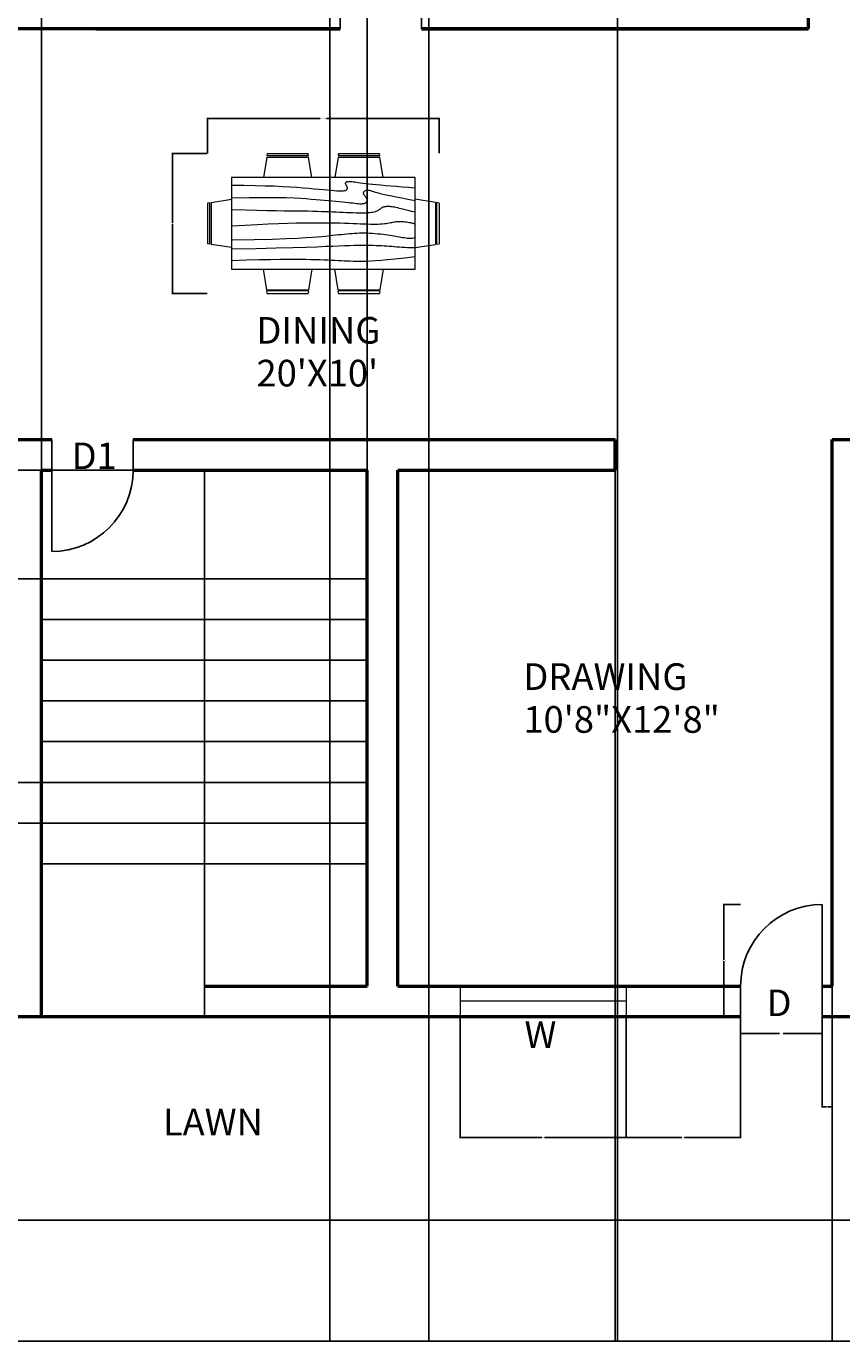
# Model space of a CAD drawing. Units: feet. Extents: x 1544 to 2324, y 1847 to 2475.
# Tile 2 of 4: x 1821 to 2061, y 1847 to 2234. Entities that reach past the tile are written whole.
import ezdxf

# ---------------------------------------------------------------- set-up
doc = ezdxf.new("R2010")
doc.units = ezdxf.units.FT
for name, color, linetype, lineweight in [('A-ANNO-DIMS', 2, 'Continuous', 18), ('A-ANNO-TEXT', 7, 'Continuous', 18), ('A-AREA-IDEN', 7, 'Continuous', 20), ('A-DOOR', 4, 'Continuous', 25), ('A-FLOR-STRS', 7, 'Continuous', 25), ('A-FURN', 8, 'Continuous', 18), ('A-GLAZ', 4, 'Continuous', 18), ('A-WALL', 7, 'Continuous', 50), ('C-PROP', 3, 'Continuous', 25)]:
    doc.layers.add(name, color=color, linetype=linetype, lineweight=lineweight)
doc.styles.get("Standard").update_dxf_attribs({"font": 'arial.ttf'})
doc.dimstyles.get("Standard").update_dxf_attribs({"dimtxt": 0.18, "dimasz": 0.18, "dimexe": 0.18, "dimexo": 0.0625, "dimgap": 0.09, "dimtad": 0, "dimtih": 1, "dimtoh": 1, "dimdec": 4, "dimzin": 0, "dimdsep": 46, "dimtxsty": 'Standard', "dimcen": 0.09, "dimadec": 0, "dimazin": 0, "dimtfac": 1, "dimtdec": 4, "dimtofl": 0, "dimtmove": 0, "dimatfit": 3, "dimfxl": 1, "dimtolj": 1, "dimtzin": 0, "dimarcsym": 0})

# ---------------------------------------------------------------- blocks, each defined once
blk = doc.blocks.new('Dining Set - 36 x 72 in.')
for p, q in [((-22.2343, 26.00059), (-23.4847, 17.99762)), ((-22.2304, 26), (-5.7608, 26)), ((-22, 27.5), (-22.1562, 26.50042)), ((-5.8416, 26.5), (-22.1534, 26.5)), ((-22, 27.5), (-6, 27.5)), ((-5.8437, 26.49966), (-6, 27.5)), ((-4.5152, 17.99762), (-5.7655, 25.99926)), ((5.7657, 26.00059), (4.5153, 17.99762)), ((5.7696, 26), (22.2392, 26)), ((6, 27.5), (5.8438, 26.50042)), ((22.1584, 26.5), (5.8466, 26.5)), ((6, 27.5), (22, 27.5)), ((22.1563, 26.49966), (22, 27.5)), ((23.4848, 17.99762), (22.2345, 25.99926)), ((36, 18), (-36, 18)), ((-36, 18), (-36, -18)), ((36, -18), (36, 18)), ((-45.5, 8), (-44.5004, 8.15617)), ((-45.5, 8), (-45.5, -8)), ((-44.5, -8.15843), (-44.5, 8.15338)), ((-44.0006, 8.23428), (-35.9976, 9.48474)), ((-44, 8.23041), (-44, -8.23915)), ((44.0006, 8.23428), (35.9976, 9.48474)), ((44, 8.23041), (44, -8.23915)), ((44.5, -8.15843), (44.5, 8.15338)), ((45.5, 8), (44.5005, 8.15617)), ((45.5, 8), (45.5, -8)), ((-44.4997, -8.15631), (-45.5, -8)), ((-35.9976, -9.48476), (-43.9993, -8.2345)), ((35.9976, -9.48476), (43.9993, -8.2345)), ((44.4997, -8.15631), (45.5, -8)), ((-36, -18), (36, -18)), ((-22.2343, -26.0006), (-23.4847, -17.99762)), ((-4.5152, -17.99762), (-5.7655, -25.99928)), ((5.7657, -26.0006), (4.5153, -17.99762)), ((23.4848, -17.99762), (22.2345, -25.99928)), ((-22.2304, -26), (-5.7608, -26)), ((-22, -27.5), (-22.1562, -26.50044)), ((-5.8416, -26.5), (-22.1534, -26.5)), ((-22, -27.5), (-6, -27.5)), ((-5.8437, -26.49967), (-6, -27.5)), ((5.7696, -26), (22.2392, -26)), ((6, -27.5), (5.8438, -26.50044)), ((22.1584, -26.5), (5.8466, -26.5)), ((6, -27.5), (22, -27.5)), ((22.1563, -26.49967), (22, -27.5))]:
    blk.add_line(p, q)
for points in [[(-36, 15), (-31.1772, 14.97754), (-26.8079, 14.91406), (-22.8538, 14.81543), (-19.276, 14.6875), (-16.0362, 14.53613), (-13.0957, 14.36718), (-10.4159, 14.18652), (-7.9583, 14), (-5.6904, 13.81315), (-3.6035, 13.63021), (-1.6954, 13.45508), (0.0365, 13.29166), (1.5945, 13.14388), (2.9811, 13.01562), (4.1988, 12.9108), (5.25, 12.83333), (6.1393, 12.78613), (6.8802, 12.76823), (7.4883, 12.77767), (7.9792, 12.8125), (8.3685, 12.87077), (8.6719, 12.95052), (8.9049, 13.0498), (9.0833, 13.16666), (9.2205, 13.29899), (9.3216, 13.44401), (9.3895, 13.59879), (9.4271, 13.76041), (9.4373, 13.92594), (9.4232, 14.09245), (9.3875, 14.257), (9.3333, 14.41666), (9.2638, 14.56917), (9.1836, 14.71484), (9.0975, 14.85465), (9.0104, 14.98958), (8.9272, 15.1206), (8.8529, 15.2487), (8.7922, 15.37483), (8.75, 15.5), (8.7305, 15.62467), (8.7344, 15.74739), (8.7617, 15.86621), (8.8125, 15.97916), (8.8867, 16.08431), (8.9844, 16.17968), (9.1055, 16.26334), (9.25, 16.33333), (9.4189, 16.38802), (9.6172, 16.42708), (9.8506, 16.45052), (10.125, 16.45833), (10.4463, 16.45052), (10.8203, 16.42708), (11.2529, 16.38802), (11.75, 16.33333), (12.3184, 16.26318), (12.9694, 16.17838), (13.7151, 16.07991), (14.5677, 15.96875), (15.5395, 15.84586), (16.6426, 15.71224), (17.8893, 15.56884), (19.2917, 15.41666), (20.859, 15.25667), (22.5879, 15.08984), (24.4721, 14.91715), (26.5052, 14.73958), (28.6809, 14.5581), (30.9929, 14.3737), (33.4347, 14.18733), (36, 14)], [(-36, 10), (-28.9766, 10.14274), (-23.1725, 10.20442), (-18.4241, 10.19775), (-14.5677, 10.13541), (-11.4399, 10.03011), (-8.877, 9.89453), (-6.7154, 9.74137), (-4.7917, 9.58333), (-2.9698, 9.43082), (-1.2246, 9.28515), (0.4415, 9.14534), (2.026, 9.01041), (3.5266, 8.87939), (4.9408, 8.7513), (6.266, 8.62516), (7.5, 8.5), (8.6411, 8.37549), (9.6914, 8.2539), (10.6538, 8.13818), (11.5312, 8.03125), (12.3267, 7.93603), (13.043, 7.85547), (13.6831, 7.79248), (14.25, 7.75), (14.7471, 7.7303), (15.1797, 7.73307), (15.5537, 7.75732), (15.875, 7.80208), (16.1494, 7.86637), (16.3828, 7.94922), (16.5811, 8.04964), (16.75, 8.16666), (16.8944, 8.29915), (17.0143, 8.44531), (17.1089, 8.60319), (17.1771, 8.77083), (17.218, 8.94629), (17.2305, 9.1276), (17.2137, 9.31282), (17.1667, 9.5), (17.0895, 9.6875), (16.987, 9.875), (16.8649, 10.0625), (16.7292, 10.25), (16.5856, 10.4375), (16.4401, 10.625), (16.2985, 10.8125), (16.1667, 11), (16.05, 11.18733), (15.9518, 11.3737), (15.8752, 11.5581), (15.8229, 11.73958), (15.798, 11.91715), (15.8034, 12.08984), (15.842, 12.25667), (15.9167, 12.41666), (16.0295, 12.56836), (16.1784, 12.70833), (16.3605, 12.83268), (16.5729, 12.9375), (16.8127, 13.01888), (17.0768, 13.07291), (17.3625, 13.0957), (17.6667, 13.08333), (17.9894, 13.03312), (18.3418, 12.94726), (18.7382, 12.82918), (19.1927, 12.68229), (19.7195, 12.51001), (20.3327, 12.31575), (21.0465, 12.10294), (21.875, 11.875), (22.8357, 11.63354), (23.959, 11.37304), (25.2786, 11.08618), (26.8282, 10.76562), (28.6414, 10.40405), (30.752, 9.99414), (33.1936, 9.52856), (36, 9)], [(-36, 5.5), (-30.7157, 5.3348), (-26.069, 5.20963), (-21.9946, 5.11767), (-18.4271, 5.05208), (-15.3009, 5.00602), (-12.5508, 4.97265), (-10.1112, 4.94515), (-7.9167, 4.91666), (-5.909, 4.88167), (-4.0586, 4.83984), (-2.3429, 4.79215), (-0.7396, 4.73958), (0.7739, 4.6831), (2.22, 4.6237), (3.6213, 4.56233), (5, 4.5), (6.373, 4.43782), (7.7344, 4.3776), (9.0723, 4.32129), (10.375, 4.27083), (11.6309, 4.22819), (12.8281, 4.19531), (13.9551, 4.17415), (15, 4.16666), (15.954, 4.17448), (16.819, 4.19791), (17.6001, 4.23698), (18.3021, 4.29166), (18.9299, 4.36198), (19.4883, 4.44791), (19.9823, 4.54948), (20.4167, 4.66666), (20.7969, 4.79899), (21.1302, 4.94401), (21.4245, 5.09879), (21.6875, 5.26041), (21.9271, 5.42594), (22.1511, 5.59245), (22.3672, 5.757), (22.5834, 5.91666), (22.8065, 6.06868), (23.0404, 6.21093), (23.2879, 6.34147), (23.5521, 6.45833), (23.8358, 6.55957), (24.142, 6.64323), (24.4735, 6.70735), (24.8334, 6.75), (25.2235, 6.76969), (25.642, 6.76692), (26.0858, 6.74267), (26.5521, 6.69791), (27.0379, 6.63362), (27.5404, 6.55078), (28.0565, 6.45036), (28.5834, 6.33333), (29.1242, 6.19987), (29.7071, 6.04687), (30.3661, 5.87044), (31.1354, 5.66666), (32.0493, 5.43164), (33.142, 5.16146), (34.4475, 4.85221), (36, 4.5)], [(-36, -1), (-30.7915, -0.6591), (-26.0195, -0.38216), (-21.6519, -0.16284), (-17.6563, 0.00521), (-14.0005, 0.12833), (-10.6523, 0.21289), (-7.5796, 0.26522), (-4.75, 0.29166), (-2.134, 0.29793), (0.2878, 0.28711), (2.5317, 0.26163), (4.6146, 0.22396), (6.5529, 0.17651), (8.3633, 0.12174), (10.0623, 0.06209), (11.6667, 0), (13.1899, -0.06201), (14.6341, -0.1211), (15.9982, -0.17432), (17.2813, -0.21875), (18.4823, -0.25147), (19.6003, -0.26953), (20.6343, -0.27002), (21.5834, -0.25), (22.4481, -0.20768), (23.2357, -0.14584), (23.9549, -0.06836), (24.6146, 0.02083), (25.2235, 0.11784), (25.7904, 0.21875), (26.3241, 0.31966), (26.8334, 0.41666), (27.3265, 0.50618), (27.8099, 0.58593), (28.2894, 0.65397), (28.7709, 0.70833), (29.2601, 0.74707), (29.763, 0.76823), (30.2855, 0.76985), (30.8334, 0.75), (31.4088, 0.70784), (31.9994, 0.64713), (32.589, 0.57275), (33.1615, 0.48958), (33.7008, 0.4025), (34.1908, 0.3164), (34.6153, 0.23616), (34.9584, 0.16666), (35.2099, 0.11165), (35.3848, 0.07031), (35.504, 0.04069), (35.5886, 0.02083), (35.6594, 0.00879), (35.7377, 0.0026), (35.8442, 0.00032), (36, 0)], [(-36, -6.5), (-27.1843, -6.31267), (-20.084, -6.1263), (-14.469, -5.9419), (-10.1094, -5.76042), (-6.7752, -5.58285), (-4.2363, -5.41016), (-2.2629, -5.24333), (-0.625, -5.08334), (0.8708, -4.93099), (2.2715, -4.78646), (3.5872, -4.64974), (4.8281, -4.52084), (6.0046, -4.39974), (7.127, -4.28646), (8.2053, -4.18099), (9.25, -4.08334), (10.2705, -3.99382), (11.2734, -3.91407), (12.2647, -3.84603), (13.25, -3.79167), (14.2354, -3.75293), (15.2266, -3.73177), (16.2295, -3.73015), (17.25, -3.75), (18.2912, -3.79248), (19.3451, -3.85547), (20.4009, -3.93604), (21.4479, -4.03125), (22.4754, -4.13819), (23.4727, -4.25391), (24.4289, -4.37549), (25.3334, -4.5), (26.1785, -4.62492), (26.9694, -4.74935), (27.7145, -4.87281), (28.4219, -4.99479), (29.1, -5.11483), (29.7572, -5.23242), (30.4016, -5.34709), (31.0417, -5.45834), (31.6837, -5.56437), (32.3262, -5.65821), (32.9658, -5.73153), (33.599, -5.77604), (34.2224, -5.78345), (34.8327, -5.74545), (35.4264, -5.65373), (36, -5.5)], [(-36, -10), (-26.4022, -9.81299), (-18.4675, -9.62891), (-11.9839, -9.45069), (-6.7396, -9.28125), (-2.5226, -9.12354), (0.8789, -8.98047), (3.6769, -8.85498), (6.0833, -8.75), (8.2767, -8.66765), (10.3021, -8.60677), (12.1712, -8.56543), (13.8958, -8.54167), (15.4876, -8.53353), (16.9583, -8.53907), (18.3197, -8.55632), (19.5834, -8.58334), (20.7616, -8.61841), (21.8685, -8.66081), (22.9188, -8.71004), (23.9271, -8.76563), (24.9081, -8.82707), (25.8763, -8.89388), (26.8465, -8.96558), (27.8334, -9.04167), (28.8474, -9.12118), (29.8828, -9.20117), (30.93, -9.27824), (31.9792, -9.34896), (33.0205, -9.40991), (34.0443, -9.45768), (35.0407, -9.48885), (36, -9.5)], [(-36, -14.5), (-30.0881, -14.33513), (-25.0332, -14.21224), (-20.7312, -14.12647), (-17.0781, -14.07292), (-13.97, -14.04671), (-11.3027, -14.04297), (-8.9724, -14.05681), (-6.875, -14.08334), (-4.9224, -14.11833), (-3.0905, -14.16016), (-1.3709, -14.20785), (0.2448, -14.26042), (1.7647, -14.3169), (3.1973, -14.3763), (4.5507, -14.43767), (5.8333, -14.5), (7.0554, -14.5621), (8.235, -14.62175), (9.3922, -14.67652), (10.5469, -14.72396), (11.7192, -14.76164), (12.929, -14.78711), (14.1965, -14.79794), (15.5417, -14.79167), (16.9933, -14.76424), (18.6152, -14.70508), (20.4804, -14.60197), (22.6615, -14.44271), (25.2312, -14.21509), (28.2624, -13.9069), (31.8277, -13.50594), (36, -13)]]:
    blk.add_lwpolyline(points)
blk = doc.blocks.new('DOOR-SINGLE-R24')
for p, q in [((9, 24), (0, 24)), ((33, 0), (0, 0))]:
    blk.add_line(p, q)
blk.add_arc((9, 0), 24, 0, 90)
blk = doc.blocks.new('*D11')
at = {"layer": 'A-ANNO-DIMS', "color": 0, "lineweight": -2, "transparency": 16777216}
for p, q in [((2031.49, 1975.67), (2026.42, 1975.67)), ((2026.6, 1975.49), (2026.6, 1959.35)), ((2026.6, 1942.85), (2026.6, 1958.99)), ((2031.49, 1942.67), (2026.42, 1942.67))]:
    blk.add_line(p, q, dxfattribs=at)
at = {"layer": 'A-ANNO-DIMS', "color": 0, "transparency": 16777216}
for points in [[(2026.57, 1975.49), (2026.63, 1975.49), (2026.6, 1975.67)], [(2026.57, 1942.85), (2026.63, 1942.85), (2026.6, 1942.67)]]:
    blk.add_solid(points, dxfattribs=at)
at = {"layer": 'Defpoints', "color": 0, "transparency": 16777216}
for p in [(2026.6, 1975.67), (2031.55, 1975.67), (2031.55, 1942.67)]:
    blk.add_point(p, dxfattribs=at)
at = {"layer": 'A-ANNO-DIMS', "color": 0, "transparency": 16777216, "insert": (2026.6, 1959.17), "char_height": 0.18, "attachment_point": 5}
blk.add_mtext('\\A1;DOOR 33 TYP.', dxfattribs=at)
blk = doc.blocks.new('*D12')
at = {"layer": 'A-ANNO-DIMS', "color": 0, "lineweight": -2, "transparency": 16777216}
for p, q in [((2031.55, 1942.61), (2031.55, 1937.54)), ((2055.55, 1942.61), (2055.55, 1937.54)), ((2031.73, 1937.72), (2043.02, 1937.72)), ((2055.37, 1937.72), (2044.08, 1937.72))]:
    blk.add_line(p, q, dxfattribs=at)
at = {"layer": 'A-ANNO-DIMS', "color": 0, "transparency": 16777216}
for points in [[(2031.73, 1937.75), (2031.73, 1937.69), (2031.55, 1937.72)], [(2055.37, 1937.75), (2055.37, 1937.69), (2055.55, 1937.72)]]:
    blk.add_solid(points, dxfattribs=at)
at = {"layer": 'Defpoints', "color": 0, "transparency": 16777216}
for p in [(2031.55, 1942.67), (2055.55, 1942.67), (2031.55, 1937.72)]:
    blk.add_point(p, dxfattribs=at)
at = {"layer": 'A-ANNO-DIMS', "color": 0, "transparency": 16777216, "insert": (2043.55, 1937.72), "char_height": 0.18, "attachment_point": 5}
blk.add_mtext('\\A1;24 TYP.', dxfattribs=at)
blk = doc.blocks.new('*D29')
at = {"layer": 'A-ANNO-DIMS', "color": 0, "lineweight": -2, "transparency": 16777216}
for p, q in [((1874.42, 2197.04), (1874.42, 2207.4)), ((1874.6, 2207.22), (1907.62, 2207.22)), ((1942.57, 2207.22), (1909.56, 2207.22)), ((1942.75, 2197.04), (1942.75, 2207.4))]:
    blk.add_line(p, q, dxfattribs=at)
at = {"layer": 'A-ANNO-DIMS', "color": 0, "transparency": 16777216}
for points in [[(1874.6, 2207.25), (1874.6, 2207.19), (1874.42, 2207.22)], [(1942.57, 2207.25), (1942.57, 2207.19), (1942.75, 2207.22)]]:
    blk.add_solid(points, dxfattribs=at)
at = {"layer": 'Defpoints', "color": 0, "transparency": 16777216}
for p in [(1942.75, 2207.22), (1874.42, 2196.97), (1942.75, 2196.97)]:
    blk.add_point(p, dxfattribs=at)
at = {"layer": 'A-ANNO-DIMS', "color": 0, "transparency": 16777216, "insert": (1908.59, 2207.22), "char_height": 0.18, "attachment_point": 5}
blk.add_mtext('\\A1;DINING SET 68', dxfattribs=at)
blk = doc.blocks.new('*D30')
at = {"layer": 'A-ANNO-DIMS', "color": 0, "lineweight": -2, "transparency": 16777216}
for p, q in [((1874.36, 2196.97), (1863.99, 2196.97)), ((1864.17, 2196.79), (1864.17, 2176.51)), ((1864.17, 2155.86), (1864.17, 2176.14)), ((1874.36, 2155.68), (1863.99, 2155.68))]:
    blk.add_line(p, q, dxfattribs=at)
at = {"layer": 'A-ANNO-DIMS', "color": 0, "transparency": 16777216}
for points in [[(1864.14, 2196.79), (1864.2, 2196.79), (1864.17, 2196.97)], [(1864.14, 2155.86), (1864.2, 2155.86), (1864.17, 2155.68)]]:
    blk.add_solid(points, dxfattribs=at)
at = {"layer": 'Defpoints', "color": 0, "transparency": 16777216}
for p in [(1864.17, 2196.97), (1874.42, 2196.97), (1874.42, 2155.68)]:
    blk.add_point(p, dxfattribs=at)
at = {"layer": 'A-ANNO-DIMS', "color": 0, "transparency": 16777216, "insert": (1864.17, 2176.33), "char_height": 0.18, "attachment_point": 5}
blk.add_mtext('\\A1;41', dxfattribs=at)
blk = doc.blocks.new('*D31')
at = {"layer": 'A-ANNO-DIMS', "color": 0, "lineweight": -2, "transparency": 16777216}
for p, q in [((1579.55, 1882.61), (1579.55, 1846.89)), ((2288.55, 1882.61), (2288.55, 1846.89)), ((1579.73, 1847.07), (1933.77, 1847.07)), ((2288.37, 1847.07), (1934.34, 1847.07))]:
    blk.add_line(p, q, dxfattribs=at)
at = {"layer": 'A-ANNO-DIMS', "color": 0, "transparency": 16777216}
for points in [[(1579.73, 1847.1), (1579.73, 1847.04), (1579.55, 1847.07)], [(2288.37, 1847.1), (2288.37, 1847.04), (2288.55, 1847.07)]]:
    blk.add_solid(points, dxfattribs=at)
at = {"layer": 'Defpoints', "color": 0, "transparency": 16777216}
for p in [(1579.55, 1882.67), (2288.55, 1882.67), (2288.55, 1847.07)]:
    blk.add_point(p, dxfattribs=at)
at = {"layer": 'A-ANNO-DIMS', "color": 0, "transparency": 16777216, "insert": (1934.05, 1847.07), "char_height": 0.18, "attachment_point": 5}
blk.add_mtext('\\A1;709', dxfattribs=at)
blk = doc.blocks.new('*D42')
at = {"layer": 'A-ANNO-DIMS', "color": 0, "lineweight": -2, "transparency": 16777216}
for p, q in [((1910.55, 2430.61), (1910.55, 1846.89)), ((1939.68, 2430.61), (1939.68, 1846.89)), ((1910.73, 1847.07), (1924.72, 1847.07)), ((1939.5, 1847.07), (1925.51, 1847.07))]:
    blk.add_line(p, q, dxfattribs=at)
at = {"layer": 'A-ANNO-DIMS', "color": 0, "transparency": 16777216}
for points in [[(1910.73, 1847.1), (1910.73, 1847.04), (1910.55, 1847.07)], [(1939.5, 1847.1), (1939.5, 1847.04), (1939.68, 1847.07)]]:
    blk.add_solid(points, dxfattribs=at)
at = {"layer": 'Defpoints', "color": 0, "transparency": 16777216}
for p in [(1910.55, 2430.67), (1939.68, 2430.67), (1939.68, 1847.07)]:
    blk.add_point(p, dxfattribs=at)
at = {"layer": 'A-ANNO-DIMS', "color": 0, "transparency": 16777216, "insert": (1925.12, 1847.07), "char_height": 0.18, "attachment_point": 5}
blk.add_mtext('\\A1;29.13', dxfattribs=at)
blk = doc.blocks.new('*D43')
at = {"layer": 'A-ANNO-DIMS', "color": 0, "lineweight": -2, "transparency": 16777216}
for p, q in [((1939.68, 2430.61), (1939.68, 1846.89)), ((1995.24, 2430.61), (1995.24, 1846.89)), ((1939.86, 1847.07), (1967.07, 1847.07)), ((1995.06, 1847.07), (1967.85, 1847.07))]:
    blk.add_line(p, q, dxfattribs=at)
at = {"layer": 'A-ANNO-DIMS', "color": 0, "transparency": 16777216}
for points in [[(1939.86, 1847.1), (1939.86, 1847.04), (1939.68, 1847.07)], [(1995.06, 1847.1), (1995.06, 1847.04), (1995.24, 1847.07)]]:
    blk.add_solid(points, dxfattribs=at)
at = {"layer": 'Defpoints', "color": 0, "transparency": 16777216}
for p in [(1939.68, 2430.67), (1995.24, 2430.67), (1995.24, 1847.07)]:
    blk.add_point(p, dxfattribs=at)
at = {"layer": 'A-ANNO-DIMS', "color": 0, "transparency": 16777216, "insert": (1967.46, 1847.07), "char_height": 0.18, "attachment_point": 5}
blk.add_mtext('\\A1;55.55', dxfattribs=at)
blk = doc.blocks.new('*D53')
at = {"layer": 'A-ANNO-DIMS', "color": 0, "lineweight": -2, "transparency": 16777216}
for p, q in [((1825.55, 2103.73), (1825.55, 2475.45)), ((1825.73, 2475.27), (1873.34, 2475.27)), ((1921.37, 2475.27), (1873.77, 2475.27)), ((1921.55, 2103.73), (1921.55, 2475.45))]:
    blk.add_line(p, q, dxfattribs=at)
at = {"layer": 'A-ANNO-DIMS', "color": 0, "transparency": 16777216}
for points in [[(1825.73, 2475.3), (1825.73, 2475.24), (1825.55, 2475.27)], [(1921.37, 2475.3), (1921.37, 2475.24), (1921.55, 2475.27)]]:
    blk.add_solid(points, dxfattribs=at)
at = {"layer": 'Defpoints', "color": 0, "transparency": 16777216}
for p in [(1921.55, 2475.27), (1825.55, 2103.67), (1921.55, 2103.67)]:
    blk.add_point(p, dxfattribs=at)
at = {"layer": 'A-ANNO-DIMS', "color": 0, "transparency": 16777216, "insert": (1873.55, 2475.27), "char_height": 0.18, "attachment_point": 5}
blk.add_mtext('\\A1;96', dxfattribs=at)
blk = doc.blocks.new('*D54')
at = {"layer": 'A-ANNO-DIMS', "color": 0, "lineweight": -2, "transparency": 16777216}
for p, q in [((1825.49, 2011.67), (1543.77, 2011.67)), ((1543.95, 2011.49), (1543.95, 2005.85)), ((1543.95, 1999.85), (1543.95, 2005.49)), ((1825.49, 1999.67), (1543.77, 1999.67))]:
    blk.add_line(p, q, dxfattribs=at)
at = {"layer": 'A-ANNO-DIMS', "color": 0, "transparency": 16777216}
for points in [[(1543.92, 2011.49), (1543.98, 2011.49), (1543.95, 2011.67)], [(1543.92, 1999.85), (1543.98, 1999.85), (1543.95, 1999.67)]]:
    blk.add_solid(points, dxfattribs=at)
at = {"layer": 'Defpoints', "color": 0, "transparency": 16777216}
for p in [(1825.55, 2011.67), (1543.95, 1999.67), (1825.55, 1999.67)]:
    blk.add_point(p, dxfattribs=at)
at = {"layer": 'A-ANNO-DIMS', "color": 0, "transparency": 16777216, "insert": (1543.95, 2005.67), "char_height": 0.18, "attachment_point": 5}
blk.add_mtext('\\A1;12', dxfattribs=at)
blk = doc.blocks.new('*D55')
at = {"layer": 'A-ANNO-DIMS', "color": 0, "lineweight": -2, "transparency": 16777216}
for p, q in [((1921.49, 2103.67), (1543.77, 2103.67)), ((1543.95, 2103.49), (1543.95, 2087.85)), ((1543.95, 2071.85), (1543.95, 2087.49)), ((1921.49, 2071.67), (1543.77, 2071.67))]:
    blk.add_line(p, q, dxfattribs=at)
at = {"layer": 'A-ANNO-DIMS', "color": 0, "transparency": 16777216}
for points in [[(1543.92, 2103.49), (1543.98, 2103.49), (1543.95, 2103.67)], [(1543.92, 2071.85), (1543.98, 2071.85), (1543.95, 2071.67)]]:
    blk.add_solid(points, dxfattribs=at)
at = {"layer": 'Defpoints', "color": 0, "transparency": 16777216}
for p in [(1543.95, 2103.67), (1921.55, 2103.67), (1921.55, 2071.67)]:
    blk.add_point(p, dxfattribs=at)
at = {"layer": 'A-ANNO-DIMS', "color": 0, "transparency": 16777216, "insert": (1543.95, 2087.67), "char_height": 0.18, "attachment_point": 5}
blk.add_mtext('\\A1;32', dxfattribs=at)
blk = doc.blocks.new('*D56')
at = {"layer": 'A-ANNO-DIMS', "color": 0, "lineweight": -2, "transparency": 16777216}
for p, q in [((2058.55, 2112.61), (2058.55, 1846.89)), ((1994.55, 2103.61), (1994.55, 1846.89)), ((1994.73, 1847.07), (2026.33, 1847.07)), ((2058.37, 1847.07), (2026.77, 1847.07))]:
    blk.add_line(p, q, dxfattribs=at)
at = {"layer": 'A-ANNO-DIMS', "color": 0, "transparency": 16777216}
for points in [[(1994.73, 1847.1), (1994.73, 1847.04), (1994.55, 1847.07)], [(2058.37, 1847.1), (2058.37, 1847.04), (2058.55, 1847.07)]]:
    blk.add_solid(points, dxfattribs=at)
at = {"layer": 'Defpoints', "color": 0, "transparency": 16777216}
for p in [(2058.55, 2112.67), (1994.55, 2103.67), (2058.55, 1847.07)]:
    blk.add_point(p, dxfattribs=at)
at = {"layer": 'A-ANNO-DIMS', "color": 0, "transparency": 16777216, "insert": (2026.55, 1847.07), "char_height": 0.18, "attachment_point": 5}
blk.add_mtext('\\A1;64', dxfattribs=at)
blk = doc.blocks.new('*D68')
at = {"layer": 'A-ANNO-DIMS', "color": 0, "lineweight": -2, "transparency": 16777216}
for p, q in [((1948.93, 1942.61), (1948.93, 1906.89)), ((1997.8, 1942.61), (1997.8, 1906.89)), ((1949.11, 1907.07), (1972.97, 1907.07)), ((1997.62, 1907.07), (1973.76, 1907.07))]:
    blk.add_line(p, q, dxfattribs=at)
at = {"layer": 'A-ANNO-DIMS', "color": 0, "transparency": 16777216}
for points in [[(1949.11, 1907.1), (1949.11, 1907.04), (1948.93, 1907.07)], [(1997.62, 1907.1), (1997.62, 1907.04), (1997.8, 1907.07)]]:
    blk.add_solid(points, dxfattribs=at)
at = {"layer": 'Defpoints', "color": 0, "transparency": 16777216}
for p in [(1948.93, 1942.67), (1997.8, 1942.67), (1948.93, 1907.07)]:
    blk.add_point(p, dxfattribs=at)
at = {"layer": 'A-ANNO-DIMS', "color": 0, "transparency": 16777216, "insert": (1973.36, 1907.07), "char_height": 0.18, "attachment_point": 5}
blk.add_mtext('\\A1;48.88', dxfattribs=at)
blk = doc.blocks.new('*D69')
at = {"layer": 'A-ANNO-DIMS', "color": 0, "lineweight": -2, "transparency": 16777216}
for p, q in [((1997.8, 1942.61), (1997.8, 1906.89)), ((2031.55, 1942.61), (2031.55, 1906.89)), ((1997.98, 1907.07), (2014.28, 1907.07)), ((2031.37, 1907.07), (2015.07, 1907.07))]:
    blk.add_line(p, q, dxfattribs=at)
at = {"layer": 'A-ANNO-DIMS', "color": 0, "transparency": 16777216}
for points in [[(1997.98, 1907.1), (1997.98, 1907.04), (1997.8, 1907.07)], [(2031.37, 1907.1), (2031.37, 1907.04), (2031.55, 1907.07)]]:
    blk.add_solid(points, dxfattribs=at)
at = {"layer": 'Defpoints', "color": 0, "transparency": 16777216}
for p in [(1997.8, 1942.67), (2031.55, 1942.67), (1997.8, 1907.07)]:
    blk.add_point(p, dxfattribs=at)
at = {"layer": 'A-ANNO-DIMS', "color": 0, "transparency": 16777216, "insert": (2014.68, 1907.07), "char_height": 0.18, "attachment_point": 5}
blk.add_mtext('\\A1;33.75', dxfattribs=at)
blk = doc.blocks.new('*D70')
at = {"layer": 'A-ANNO-DIMS', "color": 0, "lineweight": -2, "transparency": 16777216}
for p, q in [((2055.55, 1951.61), (2055.55, 1915.89)), ((2058.55, 1951.61), (2058.55, 1915.89)), ((2055.73, 1916.07), (2056.9, 1916.07)), ((2058.37, 1916.07), (2057.2, 1916.07))]:
    blk.add_line(p, q, dxfattribs=at)
at = {"layer": 'A-ANNO-DIMS', "color": 0, "transparency": 16777216}
for points in [[(2055.73, 1916.1), (2055.73, 1916.04), (2055.55, 1916.07)], [(2058.37, 1916.1), (2058.37, 1916.04), (2058.55, 1916.07)]]:
    blk.add_solid(points, dxfattribs=at)
at = {"layer": 'Defpoints', "color": 0, "transparency": 16777216}
for p in [(2055.55, 1951.67), (2058.55, 1951.67), (2055.55, 1916.07)]:
    blk.add_point(p, dxfattribs=at)
at = {"layer": 'A-ANNO-DIMS', "color": 0, "transparency": 16777216, "insert": (2057.05, 1916.07), "char_height": 0.18, "attachment_point": 5}
blk.add_mtext('\\A1;3', dxfattribs=at)

msp = doc.modelspace()

# ---------------------------------------------------------------- linework, layer by layer
at = {"layer": 'A-FLOR-STRS'}
for p, q in [((1873.5539, 1942.6692), (1873.5539, 2103.6692)), ((1825.5539, 2071.6692), (1921.5539, 2071.6692)), ((1825.5539, 2059.6692), (1921.5539, 2059.6692)), ((1825.5539, 2047.6692), (1921.5539, 2047.6692)), ((1825.5539, 2035.6692), (1921.5539, 2035.6692)), ((1825.5539, 2023.6692), (1921.5539, 2023.6692)), ((1825.5539, 2011.6692), (1921.5539, 2011.6692)), ((1825.5539, 1999.6692), (1921.5539, 1999.6692)), ((1825.5539, 1987.6692), (1921.5539, 1987.6692))]:
    msp.add_line(p, q, dxfattribs=at)
at = {"layer": 'A-GLAZ'}
for p, q in [((1948.9262, 1951.6692), (1948.9262, 1942.6692)), ((1997.803, 1951.6692), (1997.803, 1942.6692)), ((1997.803, 1947.1692), (1948.9262, 1947.1692))]:
    msp.add_line(p, q, dxfattribs=at)
at = {"layer": 'A-WALL'}
for p, q in [((2051.5539, 2233.6692), (2051.5539, 2430.6692)), ((1913.5539, 2233.6692), (1786.5539, 2233.6692)), ((1841.5539, 2233.6692), (1910.5539, 2233.6692)), ((1910.5539, 2233.6692), (1913.5539, 2233.6692)), ((2051.5539, 2233.6692), (1937.5539, 2233.6692)), ((1937.5539, 2233.6692), (2051.5539, 2233.6692)), ((1813.5539, 2112.6692), (1828.5539, 2112.6692)), ((1852.5539, 2112.6692), (1994.5539, 2112.6692)), ((1994.5539, 2103.6692), (1994.5539, 2112.6692)), ((2058.5539, 1951.6692), (2058.5539, 2112.6692)), ((2058.5539, 2112.6692), (2124.0539, 2112.6692)), ((1825.5539, 1942.6692), (1825.5539, 2103.6692)), ((1825.5539, 2103.6692), (1828.5539, 2103.6692)), ((1852.5539, 2103.6692), (1921.5539, 2103.6692)), ((1921.5539, 1951.6692), (1921.5539, 2103.6692)), ((1930.5539, 1951.6692), (1930.5539, 2103.6692)), ((1930.5539, 2103.6692), (1994.5539, 2103.6692)), ((1873.5539, 1951.6692), (1921.5539, 1951.6692)), ((1930.5539, 1951.6692), (2031.5539, 1951.6692)), ((2055.5539, 1951.6692), (2058.5539, 1951.6692)), ((1639.5539, 1942.6692), (1921.5539, 1942.6692)), ((1639.5539, 1942.6692), (2031.5539, 1942.6692)), ((2055.5539, 1942.6692), (2067.5539, 1942.6692))]:
    msp.add_line(p, q, dxfattribs=at)
at = {"layer": 'C-PROP'}
msp.add_line((1639.5539, 1882.6692), (2288.5539, 1882.6692), dxfattribs=at)

# ---------------------------------------------------------------- block references
at = {"layer": 'A-DOOR', "extrusion": (0, 0, -1), "zscale": -1, "rotation": 90.00000000000003}
msp.add_blockref('DOOR-SINGLE-R24', (-1913.5537, 2233.6693), dxfattribs=at)
at = {"layer": 'A-DOOR'}
for p, rotation in [((1828.5537, 2112.6691), 269.9999999999984), ((2055.5541, 1942.6693), 89.9999999999992)]:
    msp.add_blockref('DOOR-SINGLE-R24', p, dxfattribs=dict(at, rotation=rotation))
at = {"layer": 'A-FURN', "xscale": 0.750873874913475, "yscale": 0.750873874913475, "zscale": 0.750873874913475}
msp.add_blockref('Dining Set - 36 x 72 in.', (1908.5868, 2176.3252), dxfattribs=at)

# ---------------------------------------------------------------- texts
at = {"layer": 'A-ANNO-TEXT'}
for s, height, p in [('D1', 7.84917, (1834.4145, 2103.9336)), ('D', 7.8492, (2039.1957, 1942.7946)), ('W', 7.8492, (1967.8693, 1933.4281))]:
    msp.add_text(s, height=height, dxfattribs=at).set_placement(p)
at = {"layer": 'A-AREA-IDEN'}
for s, height, p in [('DINING', 7.84917, (1888.8867, 2140.9056)), ("20'X10'", 7.84917, (1888.8867, 2128.2966)), ('DRAWING', 7.84917, (1967.544, 2038.8909)), ('10\'8"X12\'8"', 7.849169, (1967.544, 2026.2819)), ('LAWN', 7.84917, (1861.3085, 1907.6604))]:
    msp.add_text(s, height=height, dxfattribs=at).set_placement(p)

# ---------------------------------------------------------------- dimensions: what is measured, and where the dimension line sits
at = {"layer": 'A-ANNO-DIMS'}
for base, p1, p2, override, picture, middle in [((1921.5539, 2475.2692), (1825.5539, 2103.6692), (1921.5539, 2103.6692), {"dimdec": 0, "dimlfac": 1, "dimrnd": 0, "dimzin": 0, "dimdsep": 46, "dimlunit": 2}, '*D53', (1873.5539, 2475.2692)), ((1939.6827, 1847.0692), (1910.5539, 2430.6692), (1939.6827, 2430.6692), {"dimdec": 2, "dimlfac": 1, "dimrnd": 0, "dimzin": 0, "dimdsep": 46, "dimlunit": 2}, '*D42', (1925.1183, 1847.0692)), ((1995.2363, 1847.0692), (1939.6827, 2430.6692), (1995.2363, 2430.6692), {"dimdec": 2, "dimlfac": 1, "dimrnd": 0, "dimzin": 0, "dimdsep": 46, "dimlunit": 2}, '*D43', (1967.4595, 1847.0692)), ((2058.5539, 1847.0692), (1994.5539, 2103.6692), (2058.5539, 2112.6692), {"dimdec": 0, "dimlfac": 1, "dimrnd": 0, "dimzin": 0, "dimdsep": 46, "dimlunit": 2}, '*D56', (2026.5539, 1847.0692)), ((2288.5539, 1847.0692), (1579.5539, 1882.6692), (2288.5539, 1882.6692), {"dimdec": 0, "dimlfac": 1, "dimrnd": 0, "dimzin": 0, "dimdsep": 46, "dimlunit": 2}, '*D31', (1934.0539, 1847.0692))]:
    dim = msp.add_linear_dim(base=base, p1=p1, p2=p2, dimstyle='Standard', override=override, dxfattribs=at)
    dim.commit()
    dim.dimension.update_dxf_attribs({"geometry": picture, "text_midpoint": middle})
dim = msp.add_linear_dim(base=(1942.7515, 2207.2236), p1=(1874.422, 2196.9742), p2=(1942.7515, 2196.9742), text='DINING SET <>', dimstyle='Standard', override={"dimdec": 0, "dimlfac": 1, "dimrnd": 0, "dimzin": 0, "dimdsep": 46, "dimlunit": 2}, dxfattribs=at)
dim.commit()
dim.dimension.update_dxf_attribs({"geometry": '*D29', "text_midpoint": (1908.5868, 2207.2236)})
for base, p1, p2, angle, override, picture, middle in [((1864.1726, 2196.9742), (1874.422, 2155.6762), (1874.422, 2196.9742), 90, {"dimdec": 0, "dimlfac": 1, "dimrnd": 0, "dimzin": 0, "dimdsep": 46, "dimlunit": 2}, '*D30', (1864.1726, 2176.3252)), ((1543.9539, 2103.6692), (1921.5539, 2071.6692), (1921.5539, 2103.6692), 90, {"dimdec": 0, "dimlfac": 1, "dimrnd": 0, "dimzin": 0, "dimdsep": 46, "dimlunit": 2}, '*D55', (1543.9539, 2087.6692)), ((1543.9539, 1999.6692), (1825.5539, 2011.6692), (1825.5539, 1999.6692), 90, {"dimdec": 0, "dimlfac": 1, "dimrnd": 0, "dimzin": 0, "dimdsep": 46, "dimlunit": 2}, '*D54', (1543.9539, 2005.6692)), ((2055.5539, 1916.0692), (2058.5539, 1951.6692), (2055.5539, 1951.6692), 180, {"dimdec": 0, "dimlfac": 1, "dimrnd": 0, "dimzin": 0, "dimdsep": 46, "dimlunit": 2}, '*D70', (2057.0539, 1916.0692)), ((1948.9262, 1907.0692), (1997.803, 1942.6692), (1948.9262, 1942.6692), 180, {"dimdec": 2, "dimlfac": 1, "dimrnd": 0, "dimzin": 0, "dimdsep": 46, "dimlunit": 2}, '*D68', (1973.3646, 1907.0692)), ((1997.803, 1907.0692), (2031.5539, 1942.6692), (1997.803, 1942.6692), 180, {"dimdec": 2, "dimlfac": 1, "dimrnd": 0, "dimzin": 0, "dimdsep": 46, "dimlunit": 2}, '*D69', (2014.6785, 1907.0692))]:
    dim = msp.add_linear_dim(base=base, p1=p1, p2=p2, angle=angle, dimstyle='Standard', override=override, dxfattribs=at)
    dim.commit()
    dim.dimension.update_dxf_attribs({"geometry": picture, "text_midpoint": middle})
for base, p1, p2, angle, text, picture, middle in [((2026.6039, 1975.6692), (2031.5539, 1942.6692), (2031.5539, 1975.6692), 90, 'DOOR <> TYP.', '*D11', (2026.6039, 1959.1692)), ((2031.5539, 1937.7192), (2055.5539, 1942.6692), (2031.5539, 1942.6692), 180, '<> TYP.', '*D12', (2043.5539, 1937.7192))]:
    dim = msp.add_linear_dim(base=base, p1=p1, p2=p2, angle=angle, text=text, dimstyle='Standard', override={"dimdec": 0, "dimlfac": 1, "dimrnd": 0, "dimzin": 0, "dimdsep": 46, "dimlunit": 2}, dxfattribs=at)
    dim.commit()
    dim.dimension.update_dxf_attribs({"geometry": picture, "text_midpoint": middle})

doc.saveas('drawing.dxf')
